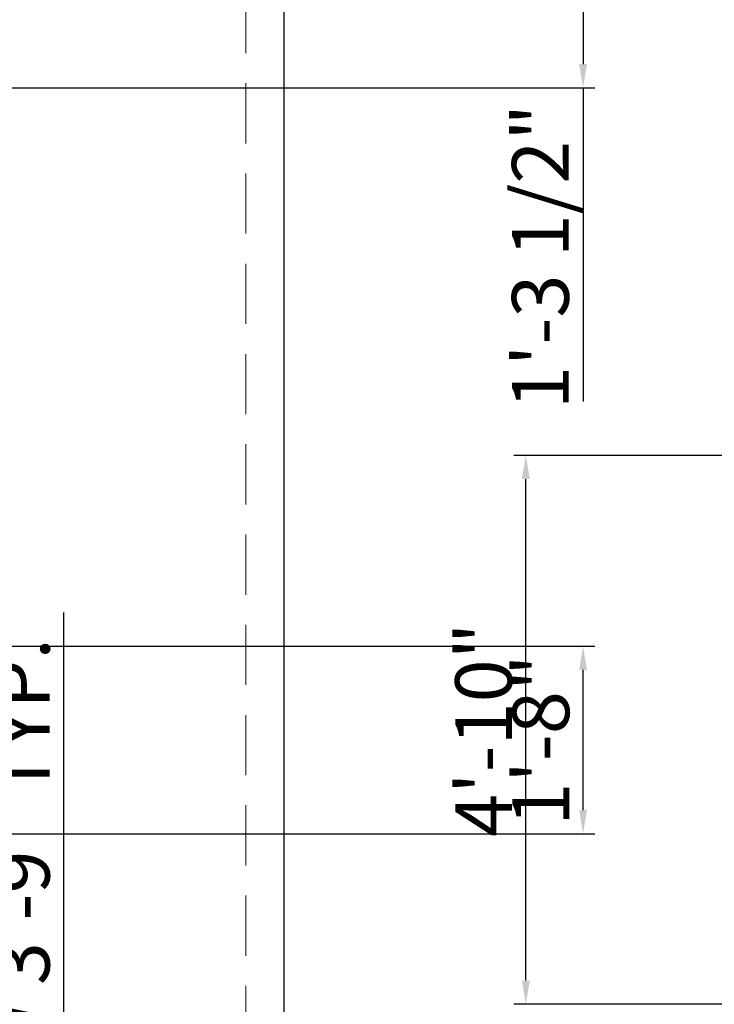
# Model space of a CAD drawing. Units: inches. Extents: x 2656 to 9931, y 1941 to 3068.
# Tile 21 of 46: x 3000 to 3074, y 2426 to 2530. Entities that reach past the tile are written whole.
import ezdxf

# ---------------------------------------------------------------- set-up
doc = ezdxf.new("R2010")
doc.units = ezdxf.units.IN
doc.linetypes.add('DASHED2', pattern=[9.525, 6.35, -3.175])
for name, color, linetype, lineweight in [('A-ANNO-DIMS', 2, 'Continuous', 18), ('A-FLOR-OVHD', 252, 'DASHED2', 13), ('C-PROP', 7, 'Continuous', 25)]:
    doc.layers.add(name, color=color, linetype=linetype, lineweight=lineweight)
doc.styles.get("Standard").update_dxf_attribs({"font": 'arial.ttf'})
doc.dimstyles.new('ISO-25', dxfattribs={"dimtxt": 6, "dimasz": 2.5, "dimexe": 1.25, "dimexo": 0.625, "dimtad": 1, "dimdec": 0, "dimlunit": 3, "dimtxsty": 'Standard', "dimcen": 2.5, "dimadec": 0, "dimazin": 0, "dimtfac": 1, "dimtdec": 0, "dimtmove": 0, "dimatfit": 3, "dimfxl": 1, "dimarcsym": 0})

# ---------------------------------------------------------------- blocks, each defined once
blk = doc.blocks.new('*D47')
at = {"layer": 'A-ANNO-DIMS', "color": 0, "lineweight": -2, "transparency": 16777216}
for p, q in [((3004.93, 2365.04), (3004.93, 2467.44)), ((2998.78, 2365.04), (3006.18, 2365.04)), ((3004.93, 2322.38), (3004.93, 2362.54)), ((2998.78, 2319.88), (3006.18, 2319.88))]:
    blk.add_line(p, q, dxfattribs=at)
at = {"layer": 'A-ANNO-DIMS', "color": 0, "transparency": 16777216}
for points in [[(3004.51, 2362.54), (3005.35, 2362.54), (3004.93, 2365.04)], [(3004.51, 2322.38), (3005.35, 2322.38), (3004.93, 2319.88)]]:
    blk.add_solid(points, dxfattribs=at)
at = {"layer": 'Defpoints', "color": 0, "transparency": 16777216}
for p in [(2998.16, 2365.04), (3004.93, 2365.04), (2998.16, 2319.88)]:
    blk.add_point(p, dxfattribs=at)
at = {"layer": 'A-ANNO-DIMS', "color": 0, "transparency": 16777216, "insert": (3001.2, 2417.49), "char_height": 6, "attachment_point": 5, "rotation": 90}
blk.add_mtext('HALL WINDOW 3\'-9" TYP.', dxfattribs=at)
blk = doc.blocks.new('*D72')
at = {"layer": 'A-ANNO-DIMS', "color": 0, "lineweight": -2, "transparency": 16777216}
for p, q in [((3144.42, 2484.03), (3052.46, 2484.03)), ((3053.71, 2428.6), (3053.71, 2481.53)), ((3144.42, 2426.1), (3052.46, 2426.1))]:
    blk.add_line(p, q, dxfattribs=at)
at = {"layer": 'A-ANNO-DIMS', "color": 0, "transparency": 16777216}
for points in [[(3053.3, 2481.53), (3054.13, 2481.53), (3053.71, 2484.03)], [(3053.3, 2428.6), (3054.13, 2428.6), (3053.71, 2426.1)]]:
    blk.add_solid(points, dxfattribs=at)
at = {"layer": 'Defpoints', "color": 0, "transparency": 16777216}
for p in [(3053.71, 2484.03), (3145.05, 2484.03), (3145.05, 2426.1)]:
    blk.add_point(p, dxfattribs=at)
at = {"layer": 'A-ANNO-DIMS', "color": 0, "transparency": 16777216, "insert": (3050.03, 2455.07), "char_height": 6, "attachment_point": 5, "rotation": 90}
blk.add_mtext('4\'-10"', dxfattribs=at)
blk = doc.blocks.new('*D75')
at = {"layer": 'A-ANNO-DIMS', "color": 0, "lineweight": -2, "transparency": 16777216}
for p, q in [((2989.78, 2463.88), (3061.01, 2463.88)), ((3059.76, 2446.6), (3059.76, 2461.38)), ((2989.78, 2444.1), (3061.01, 2444.1))]:
    blk.add_line(p, q, dxfattribs=at)
at = {"layer": 'A-ANNO-DIMS', "color": 0, "transparency": 16777216}
for points in [[(3059.34, 2461.38), (3060.17, 2461.38), (3059.76, 2463.88)], [(3059.34, 2446.6), (3060.17, 2446.6), (3059.76, 2444.1)]]:
    blk.add_solid(points, dxfattribs=at)
at = {"layer": 'Defpoints', "color": 0, "transparency": 16777216}
for p in [(2989.16, 2463.88), (3059.76, 2463.88), (2989.16, 2444.1)]:
    blk.add_point(p, dxfattribs=at)
at = {"layer": 'A-ANNO-DIMS', "color": 0, "transparency": 16777216, "insert": (3056.07, 2453.99), "char_height": 6, "attachment_point": 5, "rotation": 90}
blk.add_mtext('1\'-8"', dxfattribs=at)
blk = doc.blocks.new('*D130')
at = {"layer": 'A-ANNO-DIMS', "color": 0, "lineweight": -2, "transparency": 16777216}
for p, q in [((2877.28, 2538.52), (3061.01, 2538.52)), ((3059.76, 2536.02), (3059.76, 2525.32)), ((2902.17, 2522.82), (3061.01, 2522.82)), ((3059.76, 2522.82), (3059.76, 2489.7))]:
    blk.add_line(p, q, dxfattribs=at)
at = {"layer": 'A-ANNO-DIMS', "color": 0, "transparency": 16777216}
for points in [[(3059.34, 2536.02), (3060.17, 2536.02), (3059.76, 2538.52)], [(3059.34, 2525.32), (3060.17, 2525.32), (3059.76, 2522.82)]]:
    blk.add_solid(points, dxfattribs=at)
at = {"layer": 'Defpoints', "color": 0, "transparency": 16777216}
for p in [(2876.66, 2538.52), (2901.54, 2522.82), (3059.76, 2522.82)]:
    blk.add_point(p, dxfattribs=at)
at = {"layer": 'A-ANNO-DIMS', "color": 0, "transparency": 16777216, "insert": (3056.03, 2505.01), "char_height": 6, "attachment_point": 5, "rotation": 90}
blk.add_mtext('1\'-3 1/2"', dxfattribs=at)

msp = doc.modelspace()

# ---------------------------------------------------------------- linework, layer by layer
at = {"layer": 'A-FLOR-OVHD'}
msp.add_line((3024.16, 2637.6), (3024.16, 2090.1), dxfattribs=at)
at = {"layer": 'C-PROP'}
msp.add_line((3028.16, 2641.6), (3028.16, 2086.1), dxfattribs=at)

# ---------------------------------------------------------------- dimensions: what is measured, and where the dimension line sits
at = {"layer": 'A-ANNO-DIMS'}
for base, p1, p2, picture, middle in [((3059.76, 2522.82), (2876.66, 2538.52), (2901.54, 2522.82), '*D130', (3056.03, 2505.01)), ((3053.71, 2484.03), (3145.05, 2426.1), (3145.05, 2484.03), '*D72', (3050.03, 2455.07)), ((3059.76, 2463.88), (2989.16, 2444.1), (2989.16, 2463.88), '*D75', (3056.07, 2453.99))]:
    dim = msp.add_linear_dim(base=base, p1=p1, p2=p2, angle=90, dimstyle='ISO-25', override={"dimdec": 1, "dimlfac": 1, "dimrnd": 0, "dimzin": 1, "dimdsep": 46, "dimlunit": 4, "dimfrac": 2}, dxfattribs=at)
    dim.commit()
    dim.dimension.update_dxf_attribs({"geometry": picture, "text_midpoint": middle})
dim = msp.add_linear_dim(base=(3004.93, 2365.04), p1=(2998.16, 2319.88), p2=(2998.16, 2365.04), angle=90, text='HALL WINDOW <> TYP.', dimstyle='ISO-25', override={"dimdec": 1, "dimlfac": 1, "dimrnd": 0, "dimzin": 1, "dimdsep": 46, "dimlunit": 4, "dimfrac": 2}, dxfattribs=at)
dim.commit()
dim.dimension.update_dxf_attribs({"geometry": '*D47', "text_midpoint": (3001.2, 2417.49)})

doc.saveas('drawing.dxf')
